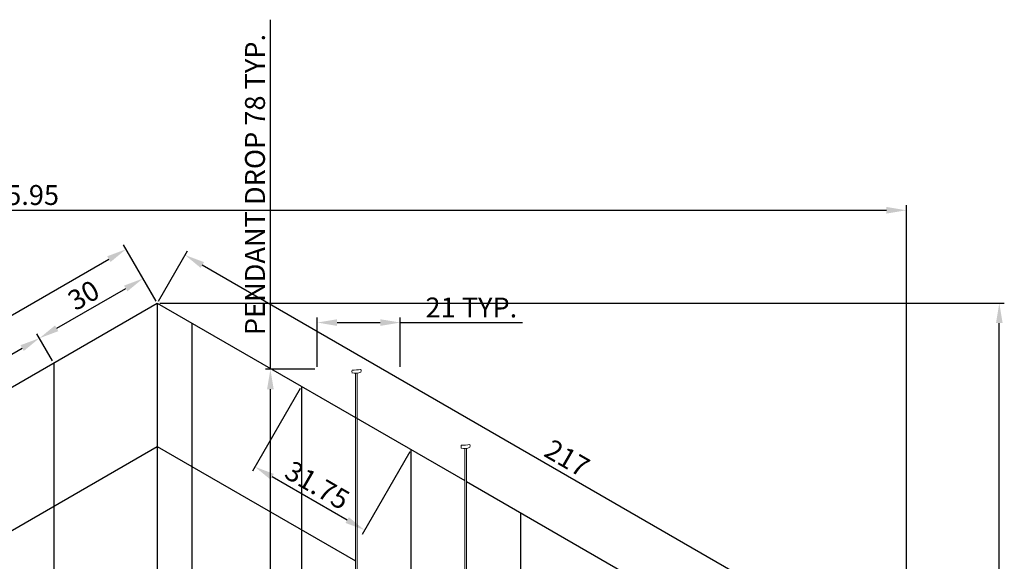
# Model space of a CAD drawing. Units: centimetres. Extents: x 2148 to 2649, y 4226 to 4785.
# Tile 6 of 6: x 2402 to 2649, y 4649 to 4785. Entities that reach past the tile are written whole.
import ezdxf

# ---------------------------------------------------------------- set-up
doc = ezdxf.new("R2010")
doc.units = ezdxf.units.CM
for name, color, linetype, lineweight in [('A-ANNO-DIMS', 63, 'Continuous', 18), ('A-ANNO-REFR', 8, 'Continuous', 13), ('A-FLOR-CASE', 21, 'Continuous', 25), ('E-LITE', 21, 'Continuous', 18)]:
    doc.layers.add(name, color=color, linetype=linetype, lineweight=lineweight)
doc.styles.get("Standard").update_dxf_attribs({"font": 'arial.ttf'})
doc.dimstyles.new('ISO-25', dxfattribs={"dimtxt": 5, "dimasz": 5, "dimexe": 1.25, "dimexo": 0.625, "dimtad": 1, "dimdec": 1, "dimtxsty": 'Standard', "dimcen": 2.5, "dimadec": 0, "dimazin": 0, "dimtfac": 1, "dimtdec": 1, "dimtmove": 0, "dimatfit": 3, "dimfxl": 1, "dimarcsym": 0})

# ---------------------------------------------------------------- blocks, each defined once
blk = doc.blocks.new('*D1')
at = {"layer": 'A-ANNO-DIMS', "color": 0, "lineweight": -2, "transparency": 16777216}
for p, q in [((2409.99, 4699.79), (2406.08, 4706.55)), ((2255.15, 4617.96), (2402.38, 4702.96)), ((2254.1, 4609.79), (2250.2, 4616.55))]:
    blk.add_line(p, q, dxfattribs=at)
at = {"layer": 'A-ANNO-DIMS', "color": 0, "transparency": 16777216}
for points in [[(2401.96, 4703.69), (2402.8, 4702.24), (2406.71, 4705.46)], [(2254.74, 4618.69), (2255.57, 4617.24), (2250.82, 4615.46)]]:
    blk.add_solid(points, dxfattribs=at)
at = {"layer": 'Defpoints', "color": 0, "transparency": 16777216}
for p in [(2406.71, 4705.46), (2410.3, 4699.24), (2254.42, 4609.24)]:
    blk.add_point(p, dxfattribs=at)
at = {"layer": 'A-ANNO-DIMS', "color": 0, "transparency": 16777216, "insert": (2327.18, 4663.22), "char_height": 5, "attachment_point": 5, "rotation": 30}
blk.add_mtext('180', dxfattribs=at)
blk = doc.blocks.new('*D2')
at = {"layer": 'A-ANNO-DIMS', "color": 0, "lineweight": -2, "transparency": 16777216}
for p, q in [((2435.97, 4714.79), (2432.08, 4721.52)), ((2411.05, 4707.94), (2428.37, 4717.94)), ((2409.99, 4699.79), (2406.1, 4706.52))]:
    blk.add_line(p, q, dxfattribs=at)
at = {"layer": 'A-ANNO-DIMS', "color": 0, "transparency": 16777216}
for points in [[(2427.96, 4718.66), (2428.79, 4717.22), (2432.7, 4720.44)], [(2410.64, 4708.66), (2411.47, 4707.22), (2406.72, 4705.44)]]:
    blk.add_solid(points, dxfattribs=at)
at = {"layer": 'Defpoints', "color": 0, "transparency": 16777216}
for p in [(2432.7, 4720.44), (2436.28, 4714.24), (2410.3, 4699.24)]:
    blk.add_point(p, dxfattribs=at)
at = {"layer": 'A-ANNO-DIMS', "color": 0, "transparency": 16777216, "insert": (2418.12, 4715.69), "char_height": 5, "attachment_point": 5, "rotation": 30}
blk.add_mtext('30', dxfattribs=at)
blk = doc.blocks.new('*D5')
at = {"layer": 'A-ANNO-DIMS', "color": 0, "lineweight": -2, "transparency": 16777216}
for p, q in [((2435.97, 4714.79), (2427.84, 4728.87)), ((2193.77, 4592.29), (2424.13, 4725.29)), ((2196.95, 4576.79), (2188.81, 4590.87))]:
    blk.add_line(p, q, dxfattribs=at)
at = {"layer": 'A-ANNO-DIMS', "color": 0, "transparency": 16777216}
for points in [[(2423.72, 4726.01), (2424.55, 4724.57), (2428.46, 4727.79)], [(2193.35, 4593.01), (2194.19, 4591.57), (2189.44, 4589.79)]]:
    blk.add_solid(points, dxfattribs=at)
at = {"layer": 'Defpoints', "color": 0, "transparency": 16777216}
for p in [(2428.46, 4727.79), (2436.28, 4714.24), (2197.26, 4576.24)]:
    blk.add_point(p, dxfattribs=at)
at = {"layer": 'A-ANNO-DIMS', "color": 0, "transparency": 16777216, "insert": (2307.36, 4661.54), "char_height": 5, "attachment_point": 5, "rotation": 30}
blk.add_mtext('276', dxfattribs=at)
blk = doc.blocks.new('*D6')
at = {"layer": 'A-ANNO-DIMS', "color": 0, "lineweight": -2, "transparency": 16777216}
for p, q in [((2436.59, 4714.79), (2443.88, 4727.41)), ((2447.59, 4723.83), (2626.86, 4620.33)), ((2624.52, 4606.29), (2631.81, 4618.91))]:
    blk.add_line(p, q, dxfattribs=at)
at = {"layer": 'A-ANNO-DIMS', "color": 0, "transparency": 16777216}
for points in [[(2448.01, 4724.55), (2447.17, 4723.11), (2443.26, 4726.33)], [(2627.27, 4621.05), (2626.44, 4619.61), (2631.19, 4617.83)]]:
    blk.add_solid(points, dxfattribs=at)
at = {"layer": 'Defpoints', "color": 0, "transparency": 16777216}
for p in [(2436.28, 4714.24), (2631.19, 4617.83), (2624.21, 4605.74)]:
    blk.add_point(p, dxfattribs=at)
at = {"layer": 'A-ANNO-DIMS', "color": 0, "transparency": 16777216, "insert": (2538.79, 4674.79), "char_height": 5, "attachment_point": 5, "rotation": 330}
blk.add_mtext('217', dxfattribs=at)
blk = doc.blocks.new('PENDANT-GLOBE')
for p, q in [((9.23, 16.63), (9.23, 76.94)), ((9.23, 16.63), (9.23, 76.94)), ((9.66, 16.72), (9.66, 76.98)), ((9.66, 16.72), (9.66, 76.98)), ((11.26, 12.41), (10.78, 15.92)), ((8.63, 11.11), (9.18, 11.2)), ((8.66, 10.87), (8.63, 11.11)), ((8.81, 9.4), (8.66, 10.87)), ((8.72, 10.24), (9.27, 10.46)), ((11.37, 11.36), (12.08, 11.47)), ((12.22, 10.56), (11.54, 10.41)), ((12.08, 11.47), (12.36, 9.65)), ((9.33, 9.46), (8.81, 9.4)), ((12.36, 9.65), (11.75, 9.55))]:
    blk.add_line(p, q)
for centre in [(8.89, 13.21), (11.04, 13.39)]:
    blk.add_circle(centre, 0.0802)
for centre, radius, start, end in [((9.99, 77.41), 1.68, 168.2535, 192.4899), ((8.39, 90.01), 12.26, 269.7881, 280.1017), ((9.16, 80.14), 3.21, 255.2356, 295.6813), ((9.7, 77.58), 0.908, 339.0828, 23.4705), ((10.08, 10.09), 10.09, 94.8735, 92.4088), ((10.25, 10.36), 2.28, 63.8319, 124.0685), ((25.64, 13.43), 14.43, 184.0611, 197.3987), ((-2.91, 9.3), 12.24, 356.9361, 13.9313), ((11.23, 5.41), 3.76, 120.6297, 80.001)]:
    blk.add_arc(centre, radius, start, end)
blk.add_ellipse((10.78, 7.32), major_axis=(0.37, -3.57), ratio=0.40259, start_param=4.289436, end_param=8.338162)
blk.add_open_spline([(8.53, 14.81), (8.46, 15.17), (8.29, 16.01), (9.68, 17.13), (10.41, 16.33), (10.78, 15.92)], degree=3, knots=[0, 0, 0, 0, 1.072444, 2.447575, 3.879684, 3.879684, 3.879684, 3.879684])
blk.add_open_spline([(8.97, 12.25), (8.82, 13.1), (8.68, 13.96), (8.53, 14.81)], degree=3)
blk = doc.blocks.new('*D26')
at = {"layer": 'A-ANNO-DIMS', "color": 0, "lineweight": -2, "transparency": 16777216}
for p, q in [((2464.67, 4697.64), (2464.67, 4785.41)), ((2475.78, 4697.64), (2463.42, 4697.64)), ((2464.67, 4624.36), (2464.67, 4692.64)), ((2475.78, 4619.36), (2463.42, 4619.36))]:
    blk.add_line(p, q, dxfattribs=at)
at = {"layer": 'A-ANNO-DIMS', "color": 0, "transparency": 16777216}
for points in [[(2463.83, 4692.64), (2465.5, 4692.64), (2464.67, 4697.64)], [(2463.83, 4624.36), (2465.5, 4624.36), (2464.67, 4619.36)]]:
    blk.add_solid(points, dxfattribs=at)
at = {"layer": 'Defpoints', "color": 0, "transparency": 16777216}
for p in [(2464.67, 4697.64), (2476.41, 4697.64), (2476.41, 4619.36)]:
    blk.add_point(p, dxfattribs=at)
at = {"layer": 'A-ANNO-DIMS', "color": 0, "transparency": 16777216, "insert": (2461.45, 4744.03), "char_height": 5, "attachment_point": 5, "rotation": 90}
blk.add_mtext('PENDANT DROP 78 TYP.', dxfattribs=at)
blk = doc.blocks.new('*D27')
at = {"layer": 'A-ANNO-DIMS', "color": 0, "lineweight": -2, "transparency": 16777216}
for p, q in [((2476.41, 4698.26), (2476.41, 4710.63)), ((2497.24, 4698.26), (2497.24, 4710.63)), ((2481.41, 4709.38), (2492.24, 4709.38)), ((2497.24, 4709.38), (2527.92, 4709.38))]:
    blk.add_line(p, q, dxfattribs=at)
at = {"layer": 'A-ANNO-DIMS', "color": 0, "transparency": 16777216}
for points in [[(2481.41, 4710.21), (2481.41, 4708.54), (2476.41, 4709.38)], [(2492.24, 4710.21), (2492.24, 4708.54), (2497.24, 4709.38)]]:
    blk.add_solid(points, dxfattribs=at)
at = {"layer": 'Defpoints', "color": 0, "transparency": 16777216}
for p in [(2497.24, 4709.38), (2476.41, 4697.64), (2497.24, 4697.64)]:
    blk.add_point(p, dxfattribs=at)
at = {"layer": 'A-ANNO-DIMS', "color": 0, "transparency": 16777216, "insert": (2515.08, 4712.51), "char_height": 5, "attachment_point": 5}
blk.add_mtext('21 TYP.', dxfattribs=at)
blk = doc.blocks.new('*D50')
at = {"layer": 'A-ANNO-DIMS', "color": 0, "lineweight": -2, "transparency": 16777216}
for p, q in [((2178.26, 4588.31), (2178.26, 4738.82)), ((2624.21, 4606.37), (2624.21, 4738.82)), ((2183.26, 4737.57), (2619.21, 4737.57))]:
    blk.add_line(p, q, dxfattribs=at)
at = {"layer": 'A-ANNO-DIMS', "color": 0, "transparency": 16777216}
for points in [[(2183.26, 4738.4), (2183.26, 4736.74), (2178.26, 4737.57)], [(2619.21, 4738.4), (2619.21, 4736.74), (2624.21, 4737.57)]]:
    blk.add_solid(points, dxfattribs=at)
at = {"layer": 'Defpoints', "color": 0, "transparency": 16777216}
for p in [(2624.21, 4737.57), (2624.21, 4605.74), (2178.26, 4587.69)]:
    blk.add_point(p, dxfattribs=at)
at = {"layer": 'A-ANNO-DIMS', "color": 0, "transparency": 16777216, "insert": (2401.23, 4740.75), "char_height": 5, "attachment_point": 5}
blk.add_mtext('445.95', dxfattribs=at)
blk = doc.blocks.new('*D51')
at = {"layer": 'A-ANNO-DIMS', "color": 0, "lineweight": -2, "transparency": 16777216}
for p, q in [((2436.91, 4714.24), (2648.78, 4714.24)), ((2647.53, 4272.37), (2647.53, 4709.24)), ((2409.81, 4267.37), (2648.78, 4267.37))]:
    blk.add_line(p, q, dxfattribs=at)
at = {"layer": 'A-ANNO-DIMS', "color": 0, "transparency": 16777216}
for points in [[(2646.7, 4709.24), (2648.37, 4709.24), (2647.53, 4714.24)], [(2646.7, 4272.37), (2648.37, 4272.37), (2647.53, 4267.37)]]:
    blk.add_solid(points, dxfattribs=at)
at = {"layer": 'Defpoints', "color": 0, "transparency": 16777216}
for p in [(2436.28, 4714.24), (2647.53, 4714.24), (2409.18, 4267.37)]:
    blk.add_point(p, dxfattribs=at)
at = {"layer": 'A-ANNO-DIMS', "color": 0, "transparency": 16777216, "insert": (2644.36, 4490.81), "char_height": 5, "attachment_point": 5, "rotation": 90}
blk.add_mtext('446.9', dxfattribs=at)
blk = doc.blocks.new('*D61')
at = {"layer": 'A-ANNO-DIMS', "color": 0, "lineweight": -2, "transparency": 16777216}
for p, q in [((2472.13, 4692.83), (2460.15, 4672.09)), ((2499.62, 4676.95), (2487.65, 4656.21)), ((2483.94, 4659.79), (2465.11, 4670.67))]:
    blk.add_line(p, q, dxfattribs=at)
at = {"layer": 'A-ANNO-DIMS', "color": 0, "transparency": 16777216}
for points in [[(2465.52, 4671.39), (2464.69, 4669.95), (2460.78, 4673.17)], [(2484.36, 4660.52), (2483.52, 4659.07), (2488.27, 4657.29)]]:
    blk.add_solid(points, dxfattribs=at)
at = {"layer": 'Defpoints', "color": 0, "transparency": 16777216}
for p in [(2472.44, 4693.37), (2499.93, 4677.49), (2460.78, 4673.17)]:
    blk.add_point(p, dxfattribs=at)
at = {"layer": 'A-ANNO-DIMS', "color": 0, "transparency": 16777216, "insert": (2476.11, 4667.99), "char_height": 5, "attachment_point": 5, "rotation": 330}
blk.add_mtext('31.75', dxfattribs=at)

msp = doc.modelspace()

# ---------------------------------------------------------------- linework, layer by layer
at = {"layer": 'A-ANNO-REFR'}
msp.add_point((2472.4377, 4657.4072), dxfattribs=at)
at = {"layer": 'A-FLOR-CASE'}
for p, q in [((2196.3921, 4575.7447), (2436.2812, 4714.2447)), ((2436.2812, 4714.2447), (2436.2812, 4606.357)), ((2436.2812, 4714.2447), (2513.4048, 4669.7174)), ((2444.9414, 4709.2447), (2444.9414, 4611.357)), ((2410.3004, 4699.2447), (2410.3004, 4529.9623)), ((2472.4377, 4693.3697), (2472.4377, 4595.482)), ((2257.0504, 4574.8032), (2436.2812, 4678.2822)), ((2436.2812, 4678.2822), (2444.9414, 4673.2822)), ((2499.934, 4677.4947), (2499.934, 4579.607)), ((2444.9414, 4673.2822), (2486.0206, 4649.5651)), ((2513.8379, 4669.4674), (2572.2471, 4635.7447)), ((2527.4303, 4661.6197), (2527.4303, 4563.732))]:
    msp.add_line(p, q, dxfattribs=at)

# ---------------------------------------------------------------- block references
at = {"layer": 'E-LITE'}
for p in [(2476.793, 4619.696), (2504.1772, 4600.8355)]:
    msp.add_blockref('PENDANT-GLOBE', p, dxfattribs=at)

# ---------------------------------------------------------------- dimensions: what is measured, and where the dimension line sits
at = {"layer": 'A-ANNO-DIMS'}
dim = msp.add_linear_dim(base=(2464.6668, 4697.6363), p1=(2476.4076, 4619.3648), p2=(2476.4076, 4697.6363), angle=90, text='PENDANT DROP <> TYP.', dimstyle='ISO-25', override={"dimdec": 0, "dimlfac": 1, "dimrnd": 0, "dimzin": 0, "dimdsep": 46, "dimlunit": 2}, dxfattribs=at)
dim.commit()
dim.dimension.update_dxf_attribs({"geometry": '*D26', "text_midpoint": (2461.4549, 4744.0253)})
dim = msp.add_linear_dim(base=(2624.2087, 4737.5697), p1=(2178.2568, 4587.6856), p2=(2624.2087, 4605.7447), dimstyle='ISO-25', override={"dimdec": 2, "dimlfac": 1, "dimrnd": 0, "dimzin": 0, "dimdsep": 46, "dimlunit": 2}, dxfattribs=at)
dim.commit()
dim.dimension.update_dxf_attribs({"geometry": '*D50', "text_midpoint": (2401.2328, 4740.7476)})
for p1, p2, distance, picture, middle in [((2197.2581, 4576.2447), (2436.2812, 4714.2447), 15.6376, '*D5', (2307.3619, 4661.5394)), ((2436.2812, 4714.2447), (2624.2087, 4605.7447), 13.9546, '*D6', (2538.7898, 4674.795)), ((2410.3004, 4699.2447), (2436.2812, 4714.2447), 7.1527, '*D2', (2418.1246, 4715.6928)), ((2254.4158, 4609.2447), (2410.3004, 4699.2447), 7.1825, '*D1', (2327.1779, 4663.217))]:
    dim = msp.add_aligned_dim(p1=p1, p2=p2, distance=distance, dimstyle='ISO-25', override={"dimclrd": 0, "dimclre": 0, "dimclrt": 0}, dxfattribs=at)
    dim.commit()
    dim.dimension.update_dxf_attribs({"geometry": picture, "text_midpoint": middle})
dim = msp.add_linear_dim(base=(2497.2428, 4709.3771), p1=(2476.4076, 4697.6363), p2=(2497.2428, 4697.6363), text='<> TYP.', dimstyle='ISO-25', override={"dimdec": 0, "dimlfac": 1, "dimrnd": 0, "dimzin": 0, "dimdsep": 46, "dimlunit": 2}, dxfattribs=at)
dim.commit()
dim.dimension.update_dxf_attribs({"geometry": '*D27', "text_midpoint": (2515.0796, 4712.514)})
for base, p1, p2, angle, override, picture, middle in [((2647.5337, 4714.2447), (2409.1829, 4267.3731), (2436.2812, 4714.2447), 90, {"dimdec": 1, "dimlfac": 1, "dimrnd": 0, "dimzin": 0, "dimdsep": 46, "dimlunit": 2}, '*D51', (2644.3558, 4490.8089)), ((2460.7752, 4673.1697), (2499.934, 4677.4947), (2472.4377, 4693.3697), 150, {"dimdec": 2, "dimlfac": 1, "dimrnd": 0, "dimzin": 0, "dimdsep": 46, "dimlunit": 2}, '*D61', (2476.1132, 4667.9858))]:
    dim = msp.add_linear_dim(base=base, p1=p1, p2=p2, angle=angle, dimstyle='ISO-25', override=override, dxfattribs=at)
    dim.commit()
    dim.dimension.update_dxf_attribs({"geometry": picture, "text_midpoint": middle})

doc.saveas('drawing.dxf')
